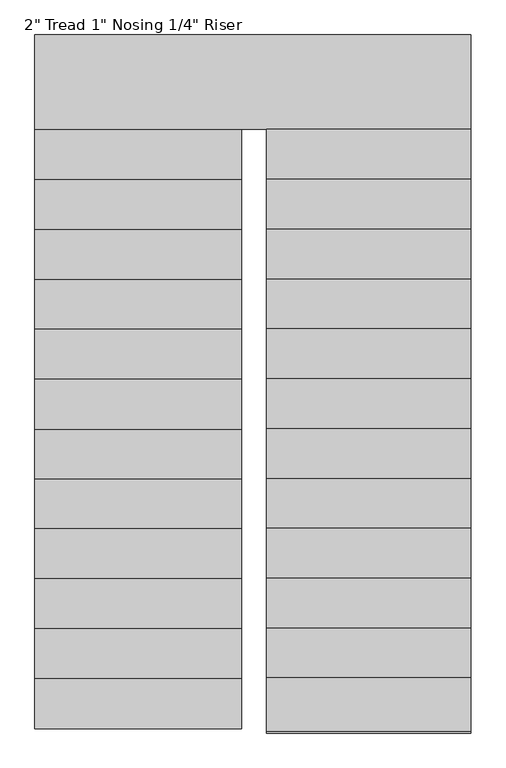
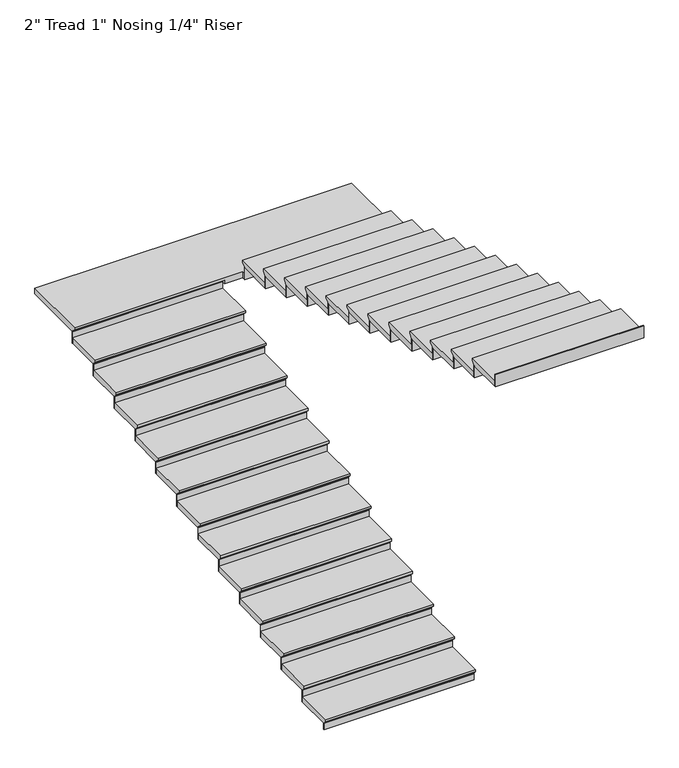
"""IFC4 building model written with IfcOpenShell, lengths in millimetres: stair flight geometry."""

from ifc_helpers import new_model, si_unit, origin, place, context, project, spatial, faceted_brep, source, transform, mapped, element, save


def stair_flight_306d97fc(model_context):
    return source(origin(), model_context, "Body", "Brep", [
        faceted_brep([(-2593.7381751, -9955.5916506, 15326.4576923), (-2593.7381751, -9955.5916506, 15345.5076923), (-3857.687215, -9955.5916506, 15345.5076923), (-3857.687215, -9955.5916506, 15326.4576923), (-2593.7381751, -9930.1916506, 15301.0576923), (-3857.687215, -9930.1916506, 15301.0576923), (-2593.7381751, -9619.0416506, 15345.5076923), (-3857.687215, -9619.0416506, 15345.5076923), (-3857.687215, -9930.1916506, 15294.7076923), (-3857.687215, -9619.0416506, 15294.7076923), (-2593.7381751, -9619.0416506, 15294.7076923), (-2593.7381751, -9930.1916506, 15294.7076923)], [[[0, 1, 2, 3]], [[4, 0, 3, 5]], [[2, 1, 6, 7]], [[8, 9, 10, 11]], [[2, 7, 9, 8, 5, 3]], [[8, 11, 4, 5]], [[6, 1, 0, 4, 11, 10]], [[7, 6, 10, 9]]]),
        faceted_brep([(-2593.7381751, -9930.1916506, 15294.7076923), (-2593.7381751, -9930.1916506, 15240.0), (-2593.7381751, -9923.8416506, 15240.0), (-2593.7381751, -9923.8416506, 15294.7076923), (-3857.687215, -9930.1916506, 15294.7076923), (-3857.687215, -9923.8416506, 15294.7076923), (-3857.687215, -9923.8416506, 15240.0), (-3857.687215, -9930.1916506, 15240.0)], [[[0, 1, 2, 3]], [[4, 5, 6, 7]], [[1, 0, 4, 7]], [[2, 1, 7, 6]], [[3, 2, 6, 5]], [[0, 3, 5, 4]]]),
        faceted_brep([(-2593.7381751, -9619.0416506, 15400.2153846), (-2593.7381751, -9619.0416506, 15294.7076923), (-2593.7381751, -9612.6916506, 15294.7076923), (-2593.7381751, -9612.6916506, 15400.2153846), (-3857.687215, -9619.0416506, 15400.2153846), (-3857.687215, -9612.6916506, 15400.2153846), (-3857.687215, -9612.6916506, 15294.7076923), (-3857.687215, -9619.0416506, 15294.7076923)], [[[0, 1, 2, 3]], [[4, 5, 6, 7]], [[1, 0, 4, 7]], [[2, 1, 7, 6]], [[3, 2, 6, 5]], [[0, 3, 5, 4]]]),
        faceted_brep([(-3857.687215, -9644.4416506, 15451.0153846), (-2593.7381751, -9644.4416506, 15451.0153846), (-2593.7381751, -9314.2416506, 15451.0153846), (-3857.687215, -9314.2416506, 15451.0153846), (-3857.687215, -9619.0416506, 15400.2153846), (-3857.687215, -9314.2416506, 15400.2153846), (-2593.7381751, -9314.2416506, 15400.2153846), (-2593.7381751, -9619.0416506, 15400.2153846), (-3857.687215, -9619.0416506, 15406.5653846), (-3857.687215, -9644.4416506, 15431.9653846), (-2593.7381751, -9619.0416506, 15406.5653846), (-2593.7381751, -9644.4416506, 15431.9653846)], [[[0, 1, 2, 3]], [[4, 5, 6, 7]], [[0, 3, 5, 4, 8, 9]], [[4, 7, 10, 8]], [[2, 1, 11, 10, 7, 6]], [[3, 2, 6, 5]], [[11, 1, 0, 9]], [[10, 11, 9, 8]]]),
        faceted_brep([(-2593.7381751, -9314.2416506, 15505.7230769), (-2593.7381751, -9314.2416506, 15400.2153846), (-2593.7381751, -9307.8916506, 15400.2153846), (-2593.7381751, -9307.8916506, 15505.7230769), (-3857.687215, -9314.2416506, 15505.7230769), (-3857.687215, -9307.8916506, 15505.7230769), (-3857.687215, -9307.8916506, 15400.2153846), (-3857.687215, -9314.2416506, 15400.2153846)], [[[0, 1, 2, 3]], [[4, 5, 6, 7]], [[1, 0, 4, 7]], [[2, 1, 7, 6]], [[3, 2, 6, 5]], [[0, 3, 5, 4]]]),
        faceted_brep([(-3857.687215, -9339.6416506, 15556.5230769), (-2593.7381751, -9339.6416506, 15556.5230769), (-2593.7381751, -9009.4416506, 15556.5230769), (-3857.687215, -9009.4416506, 15556.5230769), (-3857.687215, -9314.2416506, 15505.7230769), (-3857.687215, -9009.4416506, 15505.7230769), (-2593.7381751, -9009.4416506, 15505.7230769), (-2593.7381751, -9314.2416506, 15505.7230769), (-3857.687215, -9314.2416506, 15512.0730769), (-3857.687215, -9339.6416506, 15537.4730769), (-2593.7381751, -9314.2416506, 15512.0730769), (-2593.7381751, -9339.6416506, 15537.4730769)], [[[0, 1, 2, 3]], [[4, 5, 6, 7]], [[0, 3, 5, 4, 8, 9]], [[4, 7, 10, 8]], [[2, 1, 11, 10, 7, 6]], [[3, 2, 6, 5]], [[11, 1, 0, 9]], [[10, 11, 9, 8]]]),
        faceted_brep([(-2593.7381751, -9009.4416506, 15611.2307692), (-2593.7381751, -9009.4416506, 15505.7230769), (-2593.7381751, -9003.0916506, 15505.7230769), (-2593.7381751, -9003.0916506, 15611.2307692), (-3857.687215, -9009.4416506, 15611.2307692), (-3857.687215, -9003.0916506, 15611.2307692), (-3857.687215, -9003.0916506, 15505.7230769), (-3857.687215, -9009.4416506, 15505.7230769)], [[[0, 1, 2, 3]], [[4, 5, 6, 7]], [[1, 0, 4, 7]], [[2, 1, 7, 6]], [[3, 2, 6, 5]], [[0, 3, 5, 4]]]),
        faceted_brep([(-3857.687215, -9034.8416506, 15662.0307692), (-2593.7381751, -9034.8416506, 15662.0307692), (-2593.7381751, -8704.6416506, 15662.0307692), (-3857.687215, -8704.6416506, 15662.0307692), (-3857.687215, -9009.4416506, 15611.2307692), (-3857.687215, -8704.6416506, 15611.2307692), (-2593.7381751, -8704.6416506, 15611.2307692), (-2593.7381751, -9009.4416506, 15611.2307692), (-3857.687215, -9009.4416506, 15617.5807692), (-3857.687215, -9034.8416506, 15642.9807692), (-2593.7381751, -9009.4416506, 15617.5807692), (-2593.7381751, -9034.8416506, 15642.9807692)], [[[0, 1, 2, 3]], [[4, 5, 6, 7]], [[0, 3, 5, 4, 8, 9]], [[4, 7, 10, 8]], [[2, 1, 11, 10, 7, 6]], [[3, 2, 6, 5]], [[11, 1, 0, 9]], [[10, 11, 9, 8]]]),
        faceted_brep([(-2593.7381751, -8704.6416506, 15716.7384615), (-2593.7381751, -8704.6416506, 15611.2307692), (-2593.7381751, -8698.2916506, 15611.2307692), (-2593.7381751, -8698.2916506, 15716.7384615), (-3857.687215, -8704.6416506, 15716.7384615), (-3857.687215, -8698.2916506, 15716.7384615), (-3857.687215, -8698.2916506, 15611.2307692), (-3857.687215, -8704.6416506, 15611.2307692)], [[[0, 1, 2, 3]], [[4, 5, 6, 7]], [[1, 0, 4, 7]], [[2, 1, 7, 6]], [[3, 2, 6, 5]], [[0, 3, 5, 4]]]),
        faceted_brep([(-3857.687215, -8730.0416506, 15767.5384615), (-2593.7381751, -8730.0416506, 15767.5384615), (-2593.7381751, -8399.8416506, 15767.5384615), (-3857.687215, -8399.8416506, 15767.5384615), (-3857.687215, -8704.6416506, 15716.7384615), (-3857.687215, -8399.8416506, 15716.7384615), (-2593.7381751, -8399.8416506, 15716.7384615), (-2593.7381751, -8704.6416506, 15716.7384615), (-3857.687215, -8704.6416506, 15723.0884615), (-3857.687215, -8730.0416506, 15748.4884615), (-2593.7381751, -8704.6416506, 15723.0884615), (-2593.7381751, -8730.0416506, 15748.4884615)], [[[0, 1, 2, 3]], [[4, 5, 6, 7]], [[0, 3, 5, 4, 8, 9]], [[4, 7, 10, 8]], [[2, 1, 11, 10, 7, 6]], [[3, 2, 6, 5]], [[11, 1, 0, 9]], [[10, 11, 9, 8]]]),
        faceted_brep([(-2593.7381751, -8399.8416506, 15822.2461538), (-2593.7381751, -8399.8416506, 15716.7384615), (-2593.7381751, -8393.4916506, 15716.7384615), (-2593.7381751, -8393.4916506, 15822.2461538), (-3857.687215, -8399.8416506, 15822.2461538), (-3857.687215, -8393.4916506, 15822.2461538), (-3857.687215, -8393.4916506, 15716.7384615), (-3857.687215, -8399.8416506, 15716.7384615)], [[[0, 1, 2, 3]], [[4, 5, 6, 7]], [[1, 0, 4, 7]], [[2, 1, 7, 6]], [[3, 2, 6, 5]], [[0, 3, 5, 4]]]),
        faceted_brep([(-3857.687215, -8425.2416506, 15873.0461538), (-2593.7381751, -8425.2416506, 15873.0461538), (-2593.7381751, -8098.2166506, 15873.0461538), (-3857.687215, -8098.2166506, 15873.0461538), (-3857.687215, -8399.8416506, 15822.2461538), (-3857.687215, -8098.2166506, 15822.2461538), (-2593.7381751, -8098.2166506, 15822.2461538), (-2593.7381751, -8399.8416506, 15822.2461538), (-3857.687215, -8399.8416506, 15828.5961538), (-3857.687215, -8425.2416506, 15853.9961538), (-2593.7381751, -8399.8416506, 15828.5961538), (-2593.7381751, -8425.2416506, 15853.9961538)], [[[0, 1, 2, 3]], [[4, 5, 6, 7]], [[0, 3, 5, 4, 8, 9]], [[4, 7, 10, 8]], [[2, 1, 11, 10, 7, 6]], [[3, 2, 6, 5]], [[11, 1, 0, 9]], [[10, 11, 9, 8]]]),
        faceted_brep([(-2593.7381751, -8098.2166506, 15927.7538462), (-2593.7381751, -8098.2166506, 15822.2461538), (-2593.7381751, -8091.8666506, 15822.2461538), (-2593.7381751, -8091.8666506, 15927.7538462), (-3857.687215, -8098.2166506, 15927.7538462), (-3857.687215, -8091.8666506, 15927.7538462), (-3857.687215, -8091.8666506, 15822.2461538), (-3857.687215, -8098.2166506, 15822.2461538)], [[[0, 1, 2, 3]], [[4, 5, 6, 7]], [[1, 0, 4, 7]], [[2, 1, 7, 6]], [[3, 2, 6, 5]], [[0, 3, 5, 4]]]),
        faceted_brep([(-3857.687215, -8123.6166506, 15978.5538462), (-2593.7381751, -8123.6166506, 15978.5538462), (-2593.7381751, -7790.2416506, 15978.5538462), (-3857.687215, -7790.2416506, 15978.5538462), (-3857.687215, -8098.2166506, 15927.7538462), (-3857.687215, -7790.2416506, 15927.7538462), (-2593.7381751, -7790.2416506, 15927.7538462), (-2593.7381751, -8098.2166506, 15927.7538462), (-3857.687215, -8098.2166506, 15934.1038462), (-3857.687215, -8123.6166506, 15959.5038462), (-2593.7381751, -8098.2166506, 15934.1038462), (-2593.7381751, -8123.6166506, 15959.5038462)], [[[0, 1, 2, 3]], [[4, 5, 6, 7]], [[0, 3, 5, 4, 8, 9]], [[4, 7, 10, 8]], [[2, 1, 11, 10, 7, 6]], [[3, 2, 6, 5]], [[11, 1, 0, 9]], [[10, 11, 9, 8]]]),
        faceted_brep([(-2593.7381751, -7790.2416506, 16033.2615385), (-2593.7381751, -7790.2416506, 15927.7538462), (-2593.7381751, -7783.8916506, 15927.7538462), (-2593.7381751, -7783.8916506, 16033.2615385), (-3857.687215, -7790.2416506, 16033.2615385), (-3857.687215, -7783.8916506, 16033.2615385), (-3857.687215, -7783.8916506, 15927.7538462), (-3857.687215, -7790.2416506, 15927.7538462)], [[[0, 1, 2, 3]], [[4, 5, 6, 7]], [[1, 0, 4, 7]], [[2, 1, 7, 6]], [[3, 2, 6, 5]], [[0, 3, 5, 4]]]),
        faceted_brep([(-3857.687215, -7815.6416506, 16084.0615385), (-2593.7381751, -7815.6416506, 16084.0615385), (-2593.7381751, -7485.4416506, 16084.0615385), (-3857.687215, -7485.4416506, 16084.0615385), (-3857.687215, -7790.2416506, 16033.2615385), (-3857.687215, -7485.4416506, 16033.2615385), (-2593.7381751, -7485.4416506, 16033.2615385), (-2593.7381751, -7790.2416506, 16033.2615385), (-3857.687215, -7790.2416506, 16039.6115385), (-3857.687215, -7815.6416506, 16065.0115385), (-2593.7381751, -7790.2416506, 16039.6115385), (-2593.7381751, -7815.6416506, 16065.0115385)], [[[0, 1, 2, 3]], [[4, 5, 6, 7]], [[0, 3, 5, 4, 8, 9]], [[4, 7, 10, 8]], [[2, 1, 11, 10, 7, 6]], [[3, 2, 6, 5]], [[11, 1, 0, 9]], [[10, 11, 9, 8]]]),
        faceted_brep([(-2593.7381751, -7485.4416506, 16138.7692308), (-2593.7381751, -7485.4416506, 16033.2615385), (-2593.7381751, -7479.0916506, 16033.2615385), (-2593.7381751, -7479.0916506, 16138.7692308), (-3857.687215, -7485.4416506, 16138.7692308), (-3857.687215, -7479.0916506, 16138.7692308), (-3857.687215, -7479.0916506, 16033.2615385), (-3857.687215, -7485.4416506, 16033.2615385)], [[[0, 1, 2, 3]], [[4, 5, 6, 7]], [[1, 0, 4, 7]], [[2, 1, 7, 6]], [[3, 2, 6, 5]], [[0, 3, 5, 4]]]),
        faceted_brep([(-3857.687215, -7510.8416506, 16189.5692308), (-2593.7381751, -7510.8416506, 16189.5692308), (-2593.7381751, -7180.6416506, 16189.5692308), (-3857.687215, -7180.6416506, 16189.5692308), (-3857.687215, -7485.4416506, 16138.7692308), (-3857.687215, -7180.6416506, 16138.7692308), (-2593.7381751, -7180.6416506, 16138.7692308), (-2593.7381751, -7485.4416506, 16138.7692308), (-3857.687215, -7485.4416506, 16145.1192308), (-3857.687215, -7510.8416506, 16170.5192308), (-2593.7381751, -7485.4416506, 16145.1192308), (-2593.7381751, -7510.8416506, 16170.5192308)], [[[0, 1, 2, 3]], [[4, 5, 6, 7]], [[0, 3, 5, 4, 8, 9]], [[4, 7, 10, 8]], [[2, 1, 11, 10, 7, 6]], [[3, 2, 6, 5]], [[11, 1, 0, 9]], [[10, 11, 9, 8]]]),
        faceted_brep([(-2593.7381751, -7180.6416506, 16244.2769231), (-2593.7381751, -7180.6416506, 16138.7692308), (-2593.7381751, -7174.2916506, 16138.7692308), (-2593.7381751, -7174.2916506, 16244.2769231), (-3857.687215, -7180.6416506, 16244.2769231), (-3857.687215, -7174.2916506, 16244.2769231), (-3857.687215, -7174.2916506, 16138.7692308), (-3857.687215, -7180.6416506, 16138.7692308)], [[[0, 1, 2, 3]], [[4, 5, 6, 7]], [[1, 0, 4, 7]], [[2, 1, 7, 6]], [[3, 2, 6, 5]], [[0, 3, 5, 4]]]),
        faceted_brep([(-3857.687215, -7206.0416506, 16295.0769231), (-2593.7381751, -7206.0416506, 16295.0769231), (-2593.7381751, -6875.8416506, 16295.0769231), (-3857.687215, -6875.8416506, 16295.0769231), (-3857.687215, -7180.6416506, 16244.2769231), (-3857.687215, -6875.8416506, 16244.2769231), (-2593.7381751, -6875.8416506, 16244.2769231), (-2593.7381751, -7180.6416506, 16244.2769231), (-3857.687215, -7180.6416506, 16250.6269231), (-3857.687215, -7206.0416506, 16276.0269231), (-2593.7381751, -7180.6416506, 16250.6269231), (-2593.7381751, -7206.0416506, 16276.0269231)], [[[0, 1, 2, 3]], [[4, 5, 6, 7]], [[0, 3, 5, 4, 8, 9]], [[4, 7, 10, 8]], [[2, 1, 11, 10, 7, 6]], [[3, 2, 6, 5]], [[11, 1, 0, 9]], [[10, 11, 9, 8]]]),
        faceted_brep([(-2593.7381751, -6875.8416506, 16349.7846154), (-2593.7381751, -6875.8416506, 16244.2769231), (-2593.7381751, -6869.4916506, 16244.2769231), (-2593.7381751, -6869.4916506, 16349.7846154), (-3857.687215, -6875.8416506, 16349.7846154), (-3857.687215, -6869.4916506, 16349.7846154), (-3857.687215, -6869.4916506, 16244.2769231), (-3857.687215, -6875.8416506, 16244.2769231)], [[[0, 1, 2, 3]], [[4, 5, 6, 7]], [[1, 0, 4, 7]], [[2, 1, 7, 6]], [[3, 2, 6, 5]], [[0, 3, 5, 4]]]),
        faceted_brep([(-3857.687215, -6901.2416506, 16400.5846154), (-2593.7381751, -6901.2416506, 16400.5846154), (-2593.7381751, -6571.0416506, 16400.5846154), (-3857.687215, -6571.0416506, 16400.5846154), (-3857.687215, -6875.8416506, 16349.7846154), (-3857.687215, -6571.0416506, 16349.7846154), (-2593.7381751, -6571.0416506, 16349.7846154), (-2593.7381751, -6875.8416506, 16349.7846154), (-3857.687215, -6875.8416506, 16356.1346154), (-3857.687215, -6901.2416506, 16381.5346154), (-2593.7381751, -6875.8416506, 16356.1346154), (-2593.7381751, -6901.2416506, 16381.5346154)], [[[0, 1, 2, 3]], [[4, 5, 6, 7]], [[0, 3, 5, 4, 8, 9]], [[4, 7, 10, 8]], [[2, 1, 11, 10, 7, 6]], [[3, 2, 6, 5]], [[11, 1, 0, 9]], [[10, 11, 9, 8]]]),
        faceted_brep([(-2593.7381751, -6571.0416506, 16455.2923077), (-2593.7381751, -6571.0416506, 16349.7846154), (-2593.7381751, -6564.6916506, 16349.7846154), (-2593.7381751, -6564.6916506, 16455.2923077), (-3857.687215, -6571.0416506, 16455.2923077), (-3857.687215, -6564.6916506, 16455.2923077), (-3857.687215, -6564.6916506, 16349.7846154), (-3857.687215, -6571.0416506, 16349.7846154)], [[[0, 1, 2, 3]], [[4, 5, 6, 7]], [[1, 0, 4, 7]], [[2, 1, 7, 6]], [[3, 2, 6, 5]], [[0, 3, 5, 4]]]),
        faceted_brep([(-3857.687215, -6596.4416506, 16506.0923077), (-2593.7381751, -6596.4416506, 16506.0923077), (-2593.7381751, -6266.2416506, 16506.0923077), (-3857.687215, -6266.2416506, 16506.0923077), (-3857.687215, -6571.0416506, 16455.2923077), (-3857.687215, -6266.2416506, 16455.2923077), (-2593.7381751, -6266.2416506, 16455.2923077), (-2593.7381751, -6571.0416506, 16455.2923077), (-3857.687215, -6571.0416506, 16461.6423077), (-3857.687215, -6596.4416506, 16487.0423077), (-2593.7381751, -6571.0416506, 16461.6423077), (-2593.7381751, -6596.4416506, 16487.0423077)], [[[0, 1, 2, 3]], [[4, 5, 6, 7]], [[0, 3, 5, 4, 8, 9]], [[4, 7, 10, 8]], [[2, 1, 11, 10, 7, 6]], [[3, 2, 6, 5]], [[11, 1, 0, 9]], [[10, 11, 9, 8]]]),
        faceted_brep([(-2593.7381751, -6266.2416506, 16560.8), (-2593.7381751, -6266.2416506, 16455.2923077), (-2593.7381751, -6259.8916506, 16455.2923077), (-2593.7381751, -6259.8916506, 16560.8), (-3857.687215, -6266.2416506, 16560.8), (-3857.687215, -6259.8916506, 16560.8), (-3857.687215, -6259.8916506, 16455.2923077), (-3857.687215, -6266.2416506, 16455.2923077)], [[[0, 1, 2, 3]], [[4, 5, 6, 7]], [[1, 0, 4, 7]], [[2, 1, 7, 6]], [[3, 2, 6, 5]], [[0, 3, 5, 4]]]),
        faceted_brep([(-1190.687215, -6317.0416506, 16611.6), (-1190.687215, -5713.7916506, 16611.6), (-3857.687215, -5713.7916506, 16611.6), (-3857.687215, -6291.6416506, 16611.6), (-2441.3381751, -6291.6416506, 16611.6), (-2441.3381751, -6317.0416506, 16611.6), (-1190.687215, -5713.7916506, 16560.8), (-1190.687215, -6317.0416506, 16560.8), (-2441.3381751, -6317.0416506, 16560.8), (-2441.3381751, -6291.6416506, 16560.8), (-2593.7381751, -6291.6416506, 16560.8), (-2593.7381751, -6266.2416506, 16560.8), (-3857.687215, -6266.2416506, 16560.8), (-3857.687215, -5713.7916506, 16560.8), (-3857.687215, -6266.2416506, 16567.15), (-3857.687215, -6291.6416506, 16592.55), (-2593.7381751, -6266.2416506, 16567.15), (-2593.7381751, -6291.6416506, 16592.55)], [[[0, 1, 2, 3, 4, 5]], [[6, 7, 8, 9, 10, 11, 12, 13]], [[1, 0, 7, 6]], [[2, 1, 6, 13]], [[3, 2, 13, 12, 14, 15]], [[12, 11, 16, 14]], [[11, 10, 17, 16]], [[4, 3, 15, 17, 10, 9]], [[5, 4, 9, 8]], [[0, 5, 8, 7]], [[15, 14, 16, 17]]]),
        faceted_brep([(-2441.3381751, -6317.0416506, 16666.3076923), (-2441.3381751, -6317.0416506, 16560.8), (-2441.3381751, -6323.3916506, 16560.8), (-2441.3381751, -6323.3916506, 16666.3076923), (-1190.687215, -6317.0416506, 16666.3076923), (-1190.687215, -6323.3916506, 16666.3076923), (-1190.687215, -6323.3916506, 16560.8), (-1190.687215, -6317.0416506, 16560.8)], [[[0, 1, 2, 3]], [[4, 5, 6, 7]], [[1, 0, 4, 7]], [[2, 1, 7, 6]], [[3, 2, 6, 5]], [[0, 3, 5, 4]]]),
        faceted_brep([(-1190.687215, -6291.6416506, 16717.1076923), (-2441.3381751, -6291.6416506, 16717.1076923), (-2441.3381751, -6621.8416506, 16717.1076923), (-1190.687215, -6621.8416506, 16717.1076923), (-1190.687215, -6317.0416506, 16666.3076923), (-1190.687215, -6621.8416506, 16666.3076923), (-2441.3381751, -6621.8416506, 16666.3076923), (-2441.3381751, -6317.0416506, 16666.3076923), (-1190.687215, -6317.0416506, 16672.6576923), (-1190.687215, -6291.6416506, 16698.0576923), (-2441.3381751, -6317.0416506, 16672.6576923), (-2441.3381751, -6291.6416506, 16698.0576923)], [[[0, 1, 2, 3]], [[4, 5, 6, 7]], [[0, 3, 5, 4, 8, 9]], [[4, 7, 10, 8]], [[2, 1, 11, 10, 7, 6]], [[3, 2, 6, 5]], [[11, 1, 0, 9]], [[10, 11, 9, 8]]]),
        faceted_brep([(-2441.3381751, -6621.8416506, 16771.8153846), (-2441.3381751, -6621.8416506, 16666.3076923), (-2441.3381751, -6628.1916506, 16666.3076923), (-2441.3381751, -6628.1916506, 16771.8153846), (-1190.687215, -6621.8416506, 16771.8153846), (-1190.687215, -6628.1916506, 16771.8153846), (-1190.687215, -6628.1916506, 16666.3076923), (-1190.687215, -6621.8416506, 16666.3076923)], [[[0, 1, 2, 3]], [[4, 5, 6, 7]], [[1, 0, 4, 7]], [[2, 1, 7, 6]], [[3, 2, 6, 5]], [[0, 3, 5, 4]]]),
        faceted_brep([(-1190.687215, -6596.4416506, 16822.6153846), (-2441.3381751, -6596.4416506, 16822.6153846), (-2441.3381751, -6926.6416506, 16822.6153846), (-1190.687215, -6926.6416506, 16822.6153846), (-1190.687215, -6621.8416506, 16771.8153846), (-1190.687215, -6926.6416506, 16771.8153846), (-2441.3381751, -6926.6416506, 16771.8153846), (-2441.3381751, -6621.8416506, 16771.8153846), (-1190.687215, -6621.8416506, 16778.1653846), (-1190.687215, -6596.4416506, 16803.5653846), (-2441.3381751, -6621.8416506, 16778.1653846), (-2441.3381751, -6596.4416506, 16803.5653846)], [[[0, 1, 2, 3]], [[4, 5, 6, 7]], [[0, 3, 5, 4, 8, 9]], [[4, 7, 10, 8]], [[2, 1, 11, 10, 7, 6]], [[3, 2, 6, 5]], [[11, 1, 0, 9]], [[10, 11, 9, 8]]]),
        faceted_brep([(-2441.3381751, -6926.6416506, 16877.3230769), (-2441.3381751, -6926.6416506, 16771.8153846), (-2441.3381751, -6932.9916506, 16771.8153846), (-2441.3381751, -6932.9916506, 16877.3230769), (-1190.687215, -6926.6416506, 16877.3230769), (-1190.687215, -6932.9916506, 16877.3230769), (-1190.687215, -6932.9916506, 16771.8153846), (-1190.687215, -6926.6416506, 16771.8153846)], [[[0, 1, 2, 3]], [[4, 5, 6, 7]], [[1, 0, 4, 7]], [[2, 1, 7, 6]], [[3, 2, 6, 5]], [[0, 3, 5, 4]]]),
        faceted_brep([(-1190.687215, -6901.2416506, 16928.1230769), (-2441.3381751, -6901.2416506, 16928.1230769), (-2441.3381751, -7231.4416506, 16928.1230769), (-1190.687215, -7231.4416506, 16928.1230769), (-1190.687215, -6926.6416506, 16877.3230769), (-1190.687215, -7231.4416506, 16877.3230769), (-2441.3381751, -7231.4416506, 16877.3230769), (-2441.3381751, -6926.6416506, 16877.3230769), (-1190.687215, -6926.6416506, 16883.6730769), (-1190.687215, -6901.2416506, 16909.0730769), (-2441.3381751, -6926.6416506, 16883.6730769), (-2441.3381751, -6901.2416506, 16909.0730769)], [[[0, 1, 2, 3]], [[4, 5, 6, 7]], [[0, 3, 5, 4, 8, 9]], [[4, 7, 10, 8]], [[2, 1, 11, 10, 7, 6]], [[3, 2, 6, 5]], [[11, 1, 0, 9]], [[10, 11, 9, 8]]]),
        faceted_brep([(-2441.3381751, -7231.4416506, 16982.8307692), (-2441.3381751, -7231.4416506, 16877.3230769), (-2441.3381751, -7237.7916506, 16877.3230769), (-2441.3381751, -7237.7916506, 16982.8307692), (-1190.687215, -7231.4416506, 16982.8307692), (-1190.687215, -7237.7916506, 16982.8307692), (-1190.687215, -7237.7916506, 16877.3230769), (-1190.687215, -7231.4416506, 16877.3230769)], [[[0, 1, 2, 3]], [[4, 5, 6, 7]], [[1, 0, 4, 7]], [[2, 1, 7, 6]], [[3, 2, 6, 5]], [[0, 3, 5, 4]]]),
        faceted_brep([(-1190.687215, -7206.0416506, 17033.6307692), (-2441.3381751, -7206.0416506, 17033.6307692), (-2441.3381751, -7536.2416506, 17033.6307692), (-1190.687215, -7536.2416506, 17033.6307692), (-1190.687215, -7231.4416506, 16982.8307692), (-1190.687215, -7536.2416506, 16982.8307692), (-2441.3381751, -7536.2416506, 16982.8307692), (-2441.3381751, -7231.4416506, 16982.8307692), (-1190.687215, -7231.4416506, 16989.1807692), (-1190.687215, -7206.0416506, 17014.5807692), (-2441.3381751, -7231.4416506, 16989.1807692), (-2441.3381751, -7206.0416506, 17014.5807692)], [[[0, 1, 2, 3]], [[4, 5, 6, 7]], [[0, 3, 5, 4, 8, 9]], [[4, 7, 10, 8]], [[2, 1, 11, 10, 7, 6]], [[3, 2, 6, 5]], [[11, 1, 0, 9]], [[10, 11, 9, 8]]]),
        faceted_brep([(-2441.3381751, -7536.2416506, 17088.3384615), (-2441.3381751, -7536.2416506, 16982.8307692), (-2441.3381751, -7542.5916506, 16982.8307692), (-2441.3381751, -7542.5916506, 17088.3384615), (-1190.687215, -7536.2416506, 17088.3384615), (-1190.687215, -7542.5916506, 17088.3384615), (-1190.687215, -7542.5916506, 16982.8307692), (-1190.687215, -7536.2416506, 16982.8307692)], [[[0, 1, 2, 3]], [[4, 5, 6, 7]], [[1, 0, 4, 7]], [[2, 1, 7, 6]], [[3, 2, 6, 5]], [[0, 3, 5, 4]]]),
        faceted_brep([(-1190.687215, -7510.8416506, 17139.1384615), (-2441.3381751, -7510.8416506, 17139.1384615), (-2441.3381751, -7841.0416506, 17139.1384615), (-1190.687215, -7841.0416506, 17139.1384615), (-1190.687215, -7536.2416506, 17088.3384615), (-1190.687215, -7841.0416506, 17088.3384615), (-2441.3381751, -7841.0416506, 17088.3384615), (-2441.3381751, -7536.2416506, 17088.3384615), (-1190.687215, -7536.2416506, 17094.6884615), (-1190.687215, -7510.8416506, 17120.0884615), (-2441.3381751, -7536.2416506, 17094.6884615), (-2441.3381751, -7510.8416506, 17120.0884615)], [[[0, 1, 2, 3]], [[4, 5, 6, 7]], [[0, 3, 5, 4, 8, 9]], [[4, 7, 10, 8]], [[2, 1, 11, 10, 7, 6]], [[3, 2, 6, 5]], [[11, 1, 0, 9]], [[10, 11, 9, 8]]]),
        faceted_brep([(-2441.3381751, -7841.0416506, 17193.8461538), (-2441.3381751, -7841.0416506, 17088.3384615), (-2441.3381751, -7847.3916506, 17088.3384615), (-2441.3381751, -7847.3916506, 17193.8461538), (-1190.687215, -7841.0416506, 17193.8461538), (-1190.687215, -7847.3916506, 17193.8461538), (-1190.687215, -7847.3916506, 17088.3384615), (-1190.687215, -7841.0416506, 17088.3384615)], [[[0, 1, 2, 3]], [[4, 5, 6, 7]], [[1, 0, 4, 7]], [[2, 1, 7, 6]], [[3, 2, 6, 5]], [[0, 3, 5, 4]]]),
        faceted_brep([(-1190.687215, -7815.6416506, 17244.6461538), (-2441.3381751, -7815.6416506, 17244.6461538), (-2441.3381751, -8145.8416506, 17244.6461538), (-1190.687215, -8145.8416506, 17244.6461538), (-1190.687215, -7841.0416506, 17193.8461538), (-1190.687215, -8145.8416506, 17193.8461538), (-2441.3381751, -8145.8416506, 17193.8461538), (-2441.3381751, -7841.0416506, 17193.8461538), (-1190.687215, -7841.0416506, 17200.1961538), (-1190.687215, -7815.6416506, 17225.5961538), (-2441.3381751, -7841.0416506, 17200.1961538), (-2441.3381751, -7815.6416506, 17225.5961538)], [[[0, 1, 2, 3]], [[4, 5, 6, 7]], [[0, 3, 5, 4, 8, 9]], [[4, 7, 10, 8]], [[2, 1, 11, 10, 7, 6]], [[3, 2, 6, 5]], [[11, 1, 0, 9]], [[10, 11, 9, 8]]]),
        faceted_brep([(-2441.3381751, -8145.8416506, 17299.3538462), (-2441.3381751, -8145.8416506, 17193.8461538), (-2441.3381751, -8152.1916506, 17193.8461538), (-2441.3381751, -8152.1916506, 17299.3538462), (-1190.687215, -8145.8416506, 17299.3538462), (-1190.687215, -8152.1916506, 17299.3538462), (-1190.687215, -8152.1916506, 17193.8461538), (-1190.687215, -8145.8416506, 17193.8461538)], [[[0, 1, 2, 3]], [[4, 5, 6, 7]], [[1, 0, 4, 7]], [[2, 1, 7, 6]], [[3, 2, 6, 5]], [[0, 3, 5, 4]]]),
        faceted_brep([(-1190.687215, -8120.4416506, 17350.1538462), (-2441.3381751, -8120.4416506, 17350.1538462), (-2441.3381751, -8450.6416506, 17350.1538462), (-1190.687215, -8450.6416506, 17350.1538462), (-1190.687215, -8145.8416506, 17299.3538462), (-1190.687215, -8450.6416506, 17299.3538462), (-2441.3381751, -8450.6416506, 17299.3538462), (-2441.3381751, -8145.8416506, 17299.3538462), (-1190.687215, -8145.8416506, 17305.7038462), (-1190.687215, -8120.4416506, 17331.1038462), (-2441.3381751, -8145.8416506, 17305.7038462), (-2441.3381751, -8120.4416506, 17331.1038462)], [[[0, 1, 2, 3]], [[4, 5, 6, 7]], [[0, 3, 5, 4, 8, 9]], [[4, 7, 10, 8]], [[2, 1, 11, 10, 7, 6]], [[3, 2, 6, 5]], [[11, 1, 0, 9]], [[10, 11, 9, 8]]]),
        faceted_brep([(-2441.3381751, -8450.6416506, 17404.8615385), (-2441.3381751, -8450.6416506, 17299.3538462), (-2441.3381751, -8456.9916506, 17299.3538462), (-2441.3381751, -8456.9916506, 17404.8615385), (-1190.687215, -8450.6416506, 17404.8615385), (-1190.687215, -8456.9916506, 17404.8615385), (-1190.687215, -8456.9916506, 17299.3538462), (-1190.687215, -8450.6416506, 17299.3538462)], [[[0, 1, 2, 3]], [[4, 5, 6, 7]], [[1, 0, 4, 7]], [[2, 1, 7, 6]], [[3, 2, 6, 5]], [[0, 3, 5, 4]]]),
        faceted_brep([(-1190.687215, -8425.2416506, 17455.6615385), (-2441.3381751, -8425.2416506, 17455.6615385), (-2441.3381751, -8755.4416506, 17455.6615385), (-1190.687215, -8755.4416506, 17455.6615385), (-1190.687215, -8450.6416506, 17404.8615385), (-1190.687215, -8755.4416506, 17404.8615385), (-2441.3381751, -8755.4416506, 17404.8615385), (-2441.3381751, -8450.6416506, 17404.8615385), (-1190.687215, -8450.6416506, 17411.2115385), (-1190.687215, -8425.2416506, 17436.6115385), (-2441.3381751, -8450.6416506, 17411.2115385), (-2441.3381751, -8425.2416506, 17436.6115385)], [[[0, 1, 2, 3]], [[4, 5, 6, 7]], [[0, 3, 5, 4, 8, 9]], [[4, 7, 10, 8]], [[2, 1, 11, 10, 7, 6]], [[3, 2, 6, 5]], [[11, 1, 0, 9]], [[10, 11, 9, 8]]]),
        faceted_brep([(-2441.3381751, -8755.4416506, 17510.3692308), (-2441.3381751, -8755.4416506, 17404.8615385), (-2441.3381751, -8761.7916506, 17404.8615385), (-2441.3381751, -8761.7916506, 17510.3692308), (-1190.687215, -8755.4416506, 17510.3692308), (-1190.687215, -8761.7916506, 17510.3692308), (-1190.687215, -8761.7916506, 17404.8615385), (-1190.687215, -8755.4416506, 17404.8615385)], [[[0, 1, 2, 3]], [[4, 5, 6, 7]], [[1, 0, 4, 7]], [[2, 1, 7, 6]], [[3, 2, 6, 5]], [[0, 3, 5, 4]]]),
        faceted_brep([(-1190.687215, -8730.0416506, 17561.1692308), (-2441.3381751, -8730.0416506, 17561.1692308), (-2441.3381751, -9060.2416506, 17561.1692308), (-1190.687215, -9060.2416506, 17561.1692308), (-1190.687215, -8755.4416506, 17510.3692308), (-1190.687215, -9060.2416506, 17510.3692308), (-2441.3381751, -9060.2416506, 17510.3692308), (-2441.3381751, -8755.4416506, 17510.3692308), (-1190.687215, -8755.4416506, 17516.7192308), (-1190.687215, -8730.0416506, 17542.1192308), (-2441.3381751, -8755.4416506, 17516.7192308), (-2441.3381751, -8730.0416506, 17542.1192308)], [[[0, 1, 2, 3]], [[4, 5, 6, 7]], [[0, 3, 5, 4, 8, 9]], [[4, 7, 10, 8]], [[2, 1, 11, 10, 7, 6]], [[3, 2, 6, 5]], [[11, 1, 0, 9]], [[10, 11, 9, 8]]]),
        faceted_brep([(-2441.3381751, -9060.2416506, 17615.8769231), (-2441.3381751, -9060.2416506, 17510.3692308), (-2441.3381751, -9066.5916506, 17510.3692308), (-2441.3381751, -9066.5916506, 17615.8769231), (-1190.687215, -9060.2416506, 17615.8769231), (-1190.687215, -9066.5916506, 17615.8769231), (-1190.687215, -9066.5916506, 17510.3692308), (-1190.687215, -9060.2416506, 17510.3692308)], [[[0, 1, 2, 3]], [[4, 5, 6, 7]], [[1, 0, 4, 7]], [[2, 1, 7, 6]], [[3, 2, 6, 5]], [[0, 3, 5, 4]]]),
        faceted_brep([(-1190.687215, -9034.8416506, 17666.6769231), (-2441.3381751, -9034.8416506, 17666.6769231), (-2441.3381751, -9365.0416506, 17666.6769231), (-1190.687215, -9365.0416506, 17666.6769231), (-1190.687215, -9060.2416506, 17615.8769231), (-1190.687215, -9365.0416506, 17615.8769231), (-2441.3381751, -9365.0416506, 17615.8769231), (-2441.3381751, -9060.2416506, 17615.8769231), (-1190.687215, -9060.2416506, 17622.2269231), (-1190.687215, -9034.8416506, 17647.6269231), (-2441.3381751, -9060.2416506, 17622.2269231), (-2441.3381751, -9034.8416506, 17647.6269231)], [[[0, 1, 2, 3]], [[4, 5, 6, 7]], [[0, 3, 5, 4, 8, 9]], [[4, 7, 10, 8]], [[2, 1, 11, 10, 7, 6]], [[3, 2, 6, 5]], [[11, 1, 0, 9]], [[10, 11, 9, 8]]]),
        faceted_brep([(-2441.3381751, -9365.0416506, 17721.3846154), (-2441.3381751, -9365.0416506, 17615.8769231), (-2441.3381751, -9371.3916506, 17615.8769231), (-2441.3381751, -9371.3916506, 17721.3846154), (-1190.687215, -9365.0416506, 17721.3846154), (-1190.687215, -9371.3916506, 17721.3846154), (-1190.687215, -9371.3916506, 17615.8769231), (-1190.687215, -9365.0416506, 17615.8769231)], [[[0, 1, 2, 3]], [[4, 5, 6, 7]], [[1, 0, 4, 7]], [[2, 1, 7, 6]], [[3, 2, 6, 5]], [[0, 3, 5, 4]]]),
        faceted_brep([(-1190.687215, -9339.6416506, 17772.1846154), (-2441.3381751, -9339.6416506, 17772.1846154), (-2441.3381751, -9669.8416506, 17772.1846154), (-1190.687215, -9669.8416506, 17772.1846154), (-1190.687215, -9365.0416506, 17721.3846154), (-1190.687215, -9669.8416506, 17721.3846154), (-2441.3381751, -9669.8416506, 17721.3846154), (-2441.3381751, -9365.0416506, 17721.3846154), (-1190.687215, -9365.0416506, 17727.7346154), (-1190.687215, -9339.6416506, 17753.1346154), (-2441.3381751, -9365.0416506, 17727.7346154), (-2441.3381751, -9339.6416506, 17753.1346154)], [[[0, 1, 2, 3]], [[4, 5, 6, 7]], [[0, 3, 5, 4, 8, 9]], [[4, 7, 10, 8]], [[2, 1, 11, 10, 7, 6]], [[3, 2, 6, 5]], [[11, 1, 0, 9]], [[10, 11, 9, 8]]]),
        faceted_brep([(-2441.3381751, -9669.8416506, 17826.8923077), (-2441.3381751, -9669.8416506, 17721.3846154), (-2441.3381751, -9676.1916506, 17721.3846154), (-2441.3381751, -9676.1916506, 17826.8923077), (-1190.687215, -9669.8416506, 17826.8923077), (-1190.687215, -9676.1916506, 17826.8923077), (-1190.687215, -9676.1916506, 17721.3846154), (-1190.687215, -9669.8416506, 17721.3846154)], [[[0, 1, 2, 3]], [[4, 5, 6, 7]], [[1, 0, 4, 7]], [[2, 1, 7, 6]], [[3, 2, 6, 5]], [[0, 3, 5, 4]]]),
        faceted_brep([(-2441.3381751, -9974.6416506, 17932.4), (-2441.3381751, -9974.6416506, 17826.8923077), (-2441.3381751, -9980.9916506, 17826.8923077), (-2441.3381751, -9980.9916506, 17932.4), (-1190.687215, -9974.6416506, 17932.4), (-1190.687215, -9980.9916506, 17932.4), (-1190.687215, -9980.9916506, 17826.8923077), (-1190.687215, -9974.6416506, 17826.8923077)], [[[0, 1, 2, 3]], [[4, 5, 6, 7]], [[1, 0, 4, 7]], [[2, 1, 7, 6]], [[3, 2, 6, 5]], [[0, 3, 5, 4]]]),
        faceted_brep([(-1190.687215, -9644.4416506, 17877.6923077), (-2441.3381751, -9644.4416506, 17877.6923077), (-2441.3381751, -9974.6416506, 17877.6923077), (-1190.687215, -9974.6416506, 17877.6923077), (-1190.687215, -9669.8416506, 17826.8923077), (-1190.687215, -9974.6416506, 17826.8923077), (-2441.3381751, -9974.6416506, 17826.8923077), (-2441.3381751, -9669.8416506, 17826.8923077), (-1190.687215, -9669.8416506, 17833.2423077), (-1190.687215, -9644.4416506, 17858.6423077), (-2441.3381751, -9669.8416506, 17833.2423077), (-2441.3381751, -9644.4416506, 17858.6423077)], [[[0, 1, 2, 3]], [[4, 5, 6, 7]], [[0, 3, 5, 4, 8, 9]], [[4, 7, 10, 8]], [[2, 1, 11, 10, 7, 6]], [[3, 2, 6, 5]], [[11, 1, 0, 9]], [[10, 11, 9, 8]]]),
    ])


if __name__ == "__main__":
    model = new_model("IFC4")
    model_context = context("Model", 3, world=origin())
    ifc_project = project(units=[si_unit("LENGTHUNIT", "METRE", prefix="MILLI")], contexts=[model_context])
    site = spatial("IfcSite", under=ifc_project)
    building = spatial("IfcBuilding", under=site)
    placement = place(None, origin())
    stair_flight_shape = stair_flight_306d97fc(model_context)
    element("IfcStairFlight", 1, ObjectType="2\" Tread 1\" Nosing 1/4\" Riser", at=placement, inside=building, context=model_context, shape_type="MappedRepresentation", body=[
        mapped(stair_flight_shape, transform((0.0, 0.0, 0.0), x_axis=(1.0, 0.0, 0.0), y_axis=(0.0, 1.0, 0.0), z_axis=(0.0, 0.0, 1.0))),
    ])
    save(model, "model.ifc")
